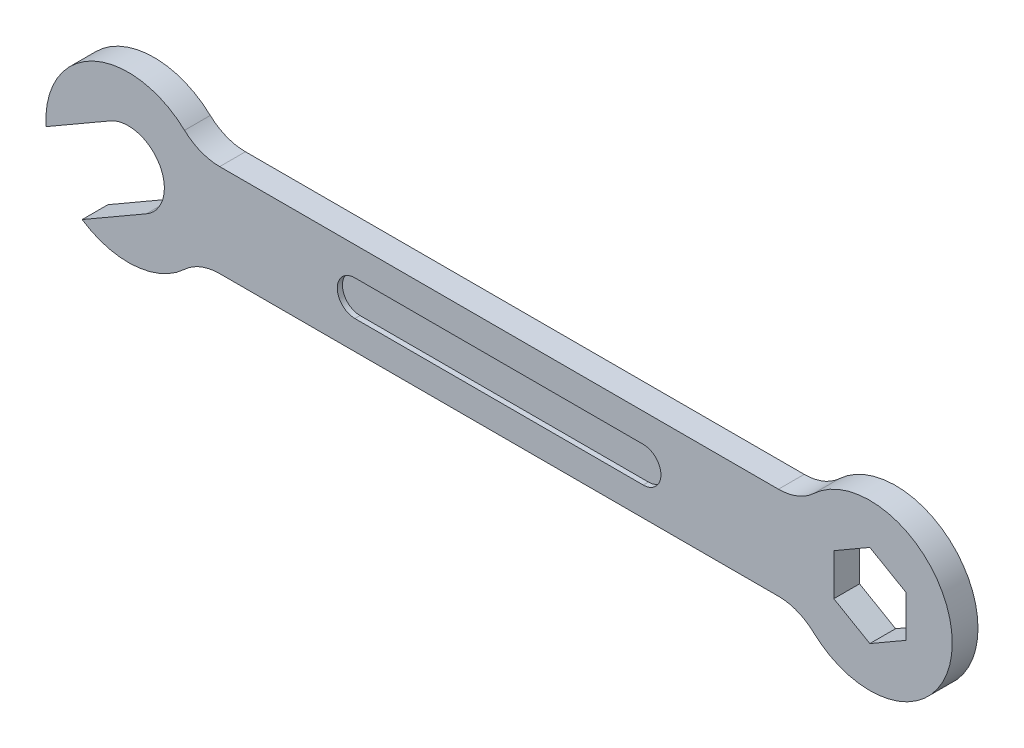
ISO-10303-21;
HEADER;
FILE_DESCRIPTION(('STEP AP214'),'2;1');
FILE_NAME('part.step','',(''),(''),'','','');
FILE_SCHEMA(('AUTOMOTIVE_DESIGN { 1 0 10303 214 1 1 1 1 }'));
ENDSEC;
DATA;
#1=APPLICATION_CONTEXT('core data for automotive mechanical design processes');
#2=APPLICATION_PROTOCOL_DEFINITION('international standard','automotive_design',2000,#1);
#3=PRODUCT_CONTEXT('',#1,'mechanical');
#4=PRODUCT('Part','Part','',(#3));
#5=PRODUCT_RELATED_PRODUCT_CATEGORY('part','',(#4));
#6=PRODUCT_DEFINITION_FORMATION('','',#4);
#7=PRODUCT_DEFINITION_CONTEXT('part definition',#1,'design');
#8=PRODUCT_DEFINITION('design','',#6,#7);
#9=PRODUCT_DEFINITION_SHAPE('','',#8);
#10=(LENGTH_UNIT() NAMED_UNIT(*) SI_UNIT(.MILLI.,.METRE.));
#11=(NAMED_UNIT(*) PLANE_ANGLE_UNIT() SI_UNIT($,.RADIAN.));
#12=(NAMED_UNIT(*) SI_UNIT($,.STERADIAN.) SOLID_ANGLE_UNIT());
#13=UNCERTAINTY_MEASURE_WITH_UNIT(LENGTH_MEASURE(1.E-05),#10,'distance_accuracy_value','');
#14=(GEOMETRIC_REPRESENTATION_CONTEXT(3) GLOBAL_UNCERTAINTY_ASSIGNED_CONTEXT((#13)) GLOBAL_UNIT_ASSIGNED_CONTEXT((#10,
#11,#12)) REPRESENTATION_CONTEXT('',''));
#15=CARTESIAN_POINT('',(0.,0.,0.));
#16=DIRECTION('',(0.,0.,1.));
#17=DIRECTION('',(1.,0.,0.));
#18=AXIS2_PLACEMENT_3D('',#15,#16,#17);
#19=CARTESIAN_POINT('',(0.,0.,2.5));
#20=DIRECTION('',(0.,0.,1.));
#21=DIRECTION('',(1.,0.,0.));
#22=AXIS2_PLACEMENT_3D('',#19,#20,#21);
#23=PLANE('',#22);
#24=CARTESIAN_POINT('',(22.,0.,2.5));
#25=DIRECTION('',(0.,0.,1.));
#26=DIRECTION('',(1.,0.,0.));
#27=AXIS2_PLACEMENT_3D('',#24,#25,#26);
#28=CIRCLE('',#27,1.71110999045574);
#29=CARTESIAN_POINT('',(22.,1.71110999045574,2.5));
#30=VERTEX_POINT('',#29);
#31=CARTESIAN_POINT('',(22.,-1.71110999045574,2.5));
#32=VERTEX_POINT('',#31);
#33=EDGE_CURVE('E53',#30,#32,#28,.T.);
#34=ORIENTED_EDGE('',*,*,#33,.F.);
#35=DIRECTION('',(-1.,0.,0.));
#36=VECTOR('',#35,1.);
#37=CARTESIAN_POINT('',(22.,1.71110999045574,2.5));
#38=LINE('',#37,#36);
#39=CARTESIAN_POINT('',(50.,1.71110999045574,2.5));
#40=VERTEX_POINT('',#39);
#41=EDGE_CURVE('E208',#40,#30,#38,.T.);
#42=ORIENTED_EDGE('',*,*,#41,.F.);
#43=CARTESIAN_POINT('',(50.,0.,2.5));
#44=DIRECTION('',(0.,0.,1.));
#45=DIRECTION('',(1.,0.,0.));
#46=AXIS2_PLACEMENT_3D('',#43,#44,#45);
#47=CIRCLE('',#46,1.71110999045574);
#48=CARTESIAN_POINT('',(50.,-1.71110999045574,2.5));
#49=VERTEX_POINT('',#48);
#50=EDGE_CURVE('E211',#49,#40,#47,.T.);
#51=ORIENTED_EDGE('',*,*,#50,.F.);
#52=DIRECTION('',(1.,0.,0.));
#53=VECTOR('',#52,1.);
#54=CARTESIAN_POINT('',(22.,-1.71110999045574,2.5));
#55=LINE('',#54,#53);
#56=EDGE_CURVE('E220',#32,#49,#55,.T.);
#57=ORIENTED_EDGE('',*,*,#56,.F.);
#58=EDGE_LOOP('',(#34,#42,#51,#57));
#59=FACE_BOUND('',#58,.T.);
#60=CARTESIAN_POINT('',(0.,0.,2.5));
#61=DIRECTION('',(0.,0.,-1.));
#62=DIRECTION('',(1.,0.,0.));
#63=AXIS2_PLACEMENT_3D('',#60,#61,#62);
#64=CIRCLE('',#63,3.5);
#65=CARTESIAN_POINT('',(-1.75,3.03108891324553,2.5));
#66=VERTEX_POINT('',#65);
#67=CARTESIAN_POINT('',(1.75,-3.03108891324553,2.5));
#68=VERTEX_POINT('',#67);
#69=EDGE_CURVE('E269',#66,#68,#64,.T.);
#70=ORIENTED_EDGE('',*,*,#69,.T.);
#71=DIRECTION('',(-0.866025403784438,-0.500000000000001,0.));
#72=VECTOR('',#71,1.);
#73=CARTESIAN_POINT('',(1.75,-3.03108891324553,2.5));
#74=LINE('',#73,#72);
#75=CARTESIAN_POINT('',(-4.47996789718855,-6.62796255573008,2.5));
#76=VERTEX_POINT('',#75);
#77=EDGE_CURVE('E272',#68,#76,#74,.T.);
#78=ORIENTED_EDGE('',*,*,#77,.T.);
#79=CARTESIAN_POINT('',(0.,0.,2.5));
#80=DIRECTION('',(0.,0.,1.));
#81=DIRECTION('',(1.,0.,0.));
#82=AXIS2_PLACEMENT_3D('',#79,#80,#81);
#83=CIRCLE('',#82,8.);
#84=CARTESIAN_POINT('',(5.46099672286118,-5.84615384615385,2.5));
#85=VERTEX_POINT('',#84);
#86=EDGE_CURVE('E277',#76,#85,#83,.T.);
#87=ORIENTED_EDGE('',*,*,#86,.T.);
#88=CARTESIAN_POINT('',(8.87411967464942,-9.5,2.5));
#89=DIRECTION('',(0.,0.,-1.));
#90=DIRECTION('',(1.,0.,0.));
#91=AXIS2_PLACEMENT_3D('',#88,#89,#90);
#92=CIRCLE('',#91,5.);
#93=CARTESIAN_POINT('',(8.87411967464942,-4.5,2.5));
#94=VERTEX_POINT('',#93);
#95=EDGE_CURVE('E279',#85,#94,#92,.T.);
#96=ORIENTED_EDGE('',*,*,#95,.T.);
#97=DIRECTION('',(1.,0.,0.));
#98=VECTOR('',#97,1.);
#99=CARTESIAN_POINT('',(8.87411967464942,-4.5,2.5));
#100=LINE('',#99,#98);
#101=CARTESIAN_POINT('',(63.1258803253506,-4.5,2.5));
#102=VERTEX_POINT('',#101);
#103=EDGE_CURVE('E278',#94,#102,#100,.T.);
#104=ORIENTED_EDGE('',*,*,#103,.T.);
#105=CARTESIAN_POINT('',(63.1258803253506,-9.50000000000001,2.5));
#106=DIRECTION('',(0.,0.,-1.));
#107=DIRECTION('',(1.,0.,0.));
#108=AXIS2_PLACEMENT_3D('',#105,#106,#107);
#109=CIRCLE('',#108,5.00000000000001);
#110=CARTESIAN_POINT('',(66.5390032771388,-5.84615384615384,2.5));
#111=VERTEX_POINT('',#110);
#112=EDGE_CURVE('E281',#102,#111,#109,.T.);
#113=ORIENTED_EDGE('',*,*,#112,.T.);
#114=CARTESIAN_POINT('',(72.,0.,2.5));
#115=DIRECTION('',(0.,0.,1.));
#116=DIRECTION('',(1.,0.,0.));
#117=AXIS2_PLACEMENT_3D('',#114,#115,#116);
#118=CIRCLE('',#117,7.99999999999999);
#119=CARTESIAN_POINT('',(66.5390032771388,5.84615384615385,2.5));
#120=VERTEX_POINT('',#119);
#121=EDGE_CURVE('E283',#111,#120,#118,.T.);
#122=ORIENTED_EDGE('',*,*,#121,.T.);
#123=CARTESIAN_POINT('',(63.1258803253506,9.50000000000001,2.5));
#124=DIRECTION('',(0.,0.,-1.));
#125=DIRECTION('',(1.,0.,0.));
#126=AXIS2_PLACEMENT_3D('',#123,#124,#125);
#127=CIRCLE('',#126,5.00000000000001);
#128=CARTESIAN_POINT('',(63.1258803253506,4.5,2.5));
#129=VERTEX_POINT('',#128);
#130=EDGE_CURVE('E289',#120,#129,#127,.T.);
#131=ORIENTED_EDGE('',*,*,#130,.T.);
#132=DIRECTION('',(-1.,0.,0.));
#133=VECTOR('',#132,1.);
#134=CARTESIAN_POINT('',(8.87411967464942,4.5,2.5));
#135=LINE('',#134,#133);
#136=CARTESIAN_POINT('',(8.87411967464942,4.5,2.5));
#137=VERTEX_POINT('',#136);
#138=EDGE_CURVE('E290',#129,#137,#135,.T.);
#139=ORIENTED_EDGE('',*,*,#138,.T.);
#140=CARTESIAN_POINT('',(8.87411967464942,9.5,2.5));
#141=DIRECTION('',(0.,0.,-1.));
#142=DIRECTION('',(1.,0.,0.));
#143=AXIS2_PLACEMENT_3D('',#140,#141,#142);
#144=CIRCLE('',#143,5.);
#145=CARTESIAN_POINT('',(5.46099672286118,5.84615384615385,2.5));
#146=VERTEX_POINT('',#145);
#147=EDGE_CURVE('E287',#137,#146,#144,.T.);
#148=ORIENTED_EDGE('',*,*,#147,.T.);
#149=CARTESIAN_POINT('',(0.,0.,2.5));
#150=DIRECTION('',(0.,0.,1.));
#151=DIRECTION('',(1.,0.,0.));
#152=AXIS2_PLACEMENT_3D('',#149,#150,#151);
#153=CIRCLE('',#152,8.);
#154=CARTESIAN_POINT('',(-7.97996789718856,-0.565784729239017,2.5));
#155=VERTEX_POINT('',#154);
#156=EDGE_CURVE('E295',#146,#155,#153,.T.);
#157=ORIENTED_EDGE('',*,*,#156,.T.);
#158=DIRECTION('',(0.866025403784438,0.500000000000001,0.));
#159=VECTOR('',#158,1.);
#160=CARTESIAN_POINT('',(-1.75,3.03108891324553,2.5));
#161=LINE('',#160,#159);
#162=EDGE_CURVE('E294',#155,#66,#161,.T.);
#163=ORIENTED_EDGE('',*,*,#162,.T.);
#164=EDGE_LOOP('',(#70,#78,#87,#96,#104,#113,#122,#131,#139,#148,#157,#163));
#165=FACE_BOUND('',#164,.T.);
#166=DIRECTION('',(0.,1.,0.));
#167=VECTOR('',#166,1.);
#168=CARTESIAN_POINT('',(75.5,-2.02072594216369,2.5));
#169=LINE('',#168,#167);
#170=CARTESIAN_POINT('',(75.5,-2.02072594216369,2.5));
#171=VERTEX_POINT('',#170);
#172=CARTESIAN_POINT('',(75.5,2.02072594216369,2.5));
#173=VERTEX_POINT('',#172);
#174=EDGE_CURVE('E228',#171,#173,#169,.T.);
#175=ORIENTED_EDGE('',*,*,#174,.F.);
#176=DIRECTION('',(0.866025403784438,0.5,0.));
#177=VECTOR('',#176,1.);
#178=CARTESIAN_POINT('',(72.,-4.04145188432738,2.5));
#179=LINE('',#178,#177);
#180=CARTESIAN_POINT('',(72.,-4.04145188432738,2.5));
#181=VERTEX_POINT('',#180);
#182=EDGE_CURVE('E226',#181,#171,#179,.T.);
#183=ORIENTED_EDGE('',*,*,#182,.F.);
#184=DIRECTION('',(0.866025403784439,-0.5,0.));
#185=VECTOR('',#184,1.);
#186=CARTESIAN_POINT('',(68.5,-2.02072594216369,2.5));
#187=LINE('',#186,#185);
#188=CARTESIAN_POINT('',(68.5,-2.02072594216369,2.5));
#189=VERTEX_POINT('',#188);
#190=EDGE_CURVE('E236',#189,#181,#187,.T.);
#191=ORIENTED_EDGE('',*,*,#190,.F.);
#192=DIRECTION('',(0.,-1.,0.));
#193=VECTOR('',#192,1.);
#194=CARTESIAN_POINT('',(68.5,2.02072594216368,2.5));
#195=LINE('',#194,#193);
#196=CARTESIAN_POINT('',(68.5,2.02072594216368,2.5));
#197=VERTEX_POINT('',#196);
#198=EDGE_CURVE('E237',#197,#189,#195,.T.);
#199=ORIENTED_EDGE('',*,*,#198,.F.);
#200=DIRECTION('',(-0.866025403784438,-0.5,0.));
#201=VECTOR('',#200,1.);
#202=CARTESIAN_POINT('',(72.,4.04145188432738,2.5));
#203=LINE('',#202,#201);
#204=CARTESIAN_POINT('',(72.,4.04145188432738,2.5));
#205=VERTEX_POINT('',#204);
#206=EDGE_CURVE('E233',#205,#197,#203,.T.);
#207=ORIENTED_EDGE('',*,*,#206,.F.);
#208=DIRECTION('',(-0.866025403784439,0.5,0.));
#209=VECTOR('',#208,1.);
#210=CARTESIAN_POINT('',(75.5,2.02072594216369,2.5));
#211=LINE('',#210,#209);
#212=EDGE_CURVE('E231',#173,#205,#211,.T.);
#213=ORIENTED_EDGE('',*,*,#212,.F.);
#214=EDGE_LOOP('',(#175,#183,#191,#199,#207,#213));
#215=FACE_BOUND('',#214,.T.);
#216=ADVANCED_FACE('F39',(#59,#165,#215),#23,.T.);
#217=CARTESIAN_POINT('',(0.,0.,0.));
#218=DIRECTION('',(0.,0.,1.));
#219=DIRECTION('',(1.,0.,0.));
#220=AXIS2_PLACEMENT_3D('',#217,#218,#219);
#221=PLANE('',#220);
#222=CARTESIAN_POINT('',(0.,0.,0.));
#223=DIRECTION('',(0.,0.,-1.));
#224=DIRECTION('',(1.,0.,0.));
#225=AXIS2_PLACEMENT_3D('',#222,#223,#224);
#226=CIRCLE('',#225,3.5);
#227=CARTESIAN_POINT('',(-1.75,3.03108891324553,0.));
#228=VERTEX_POINT('',#227);
#229=CARTESIAN_POINT('',(1.75,-3.03108891324553,0.));
#230=VERTEX_POINT('',#229);
#231=EDGE_CURVE('E267',#228,#230,#226,.T.);
#232=ORIENTED_EDGE('',*,*,#231,.F.);
#233=DIRECTION('',(0.866025403784438,0.500000000000001,0.));
#234=VECTOR('',#233,1.);
#235=CARTESIAN_POINT('',(-1.75,3.03108891324553,0.));
#236=LINE('',#235,#234);
#237=CARTESIAN_POINT('',(-7.97996789718856,-0.565784729239017,0.));
#238=VERTEX_POINT('',#237);
#239=EDGE_CURVE('E273',#238,#228,#236,.T.);
#240=ORIENTED_EDGE('',*,*,#239,.F.);
#241=CARTESIAN_POINT('',(0.,0.,0.));
#242=DIRECTION('',(0.,0.,1.));
#243=DIRECTION('',(1.,0.,0.));
#244=AXIS2_PLACEMENT_3D('',#241,#242,#243);
#245=CIRCLE('',#244,8.);
#246=CARTESIAN_POINT('',(5.46099672286118,5.84615384615385,0.));
#247=VERTEX_POINT('',#246);
#248=EDGE_CURVE('E320',#247,#238,#245,.T.);
#249=ORIENTED_EDGE('',*,*,#248,.F.);
#250=CARTESIAN_POINT('',(8.87411967464942,9.5,0.));
#251=DIRECTION('',(0.,0.,-1.));
#252=DIRECTION('',(1.,0.,0.));
#253=AXIS2_PLACEMENT_3D('',#250,#251,#252);
#254=CIRCLE('',#253,5.);
#255=CARTESIAN_POINT('',(8.87411967464942,4.5,0.));
#256=VERTEX_POINT('',#255);
#257=EDGE_CURVE('E312',#256,#247,#254,.T.);
#258=ORIENTED_EDGE('',*,*,#257,.F.);
#259=DIRECTION('',(-1.,0.,0.));
#260=VECTOR('',#259,1.);
#261=CARTESIAN_POINT('',(8.87411967464942,4.5,0.));
#262=LINE('',#261,#260);
#263=CARTESIAN_POINT('',(63.1258803253506,4.5,0.));
#264=VERTEX_POINT('',#263);
#265=EDGE_CURVE('E311',#264,#256,#262,.T.);
#266=ORIENTED_EDGE('',*,*,#265,.F.);
#267=CARTESIAN_POINT('',(63.1258803253506,9.50000000000001,0.));
#268=DIRECTION('',(0.,0.,-1.));
#269=DIRECTION('',(1.,0.,0.));
#270=AXIS2_PLACEMENT_3D('',#267,#268,#269);
#271=CIRCLE('',#270,5.00000000000001);
#272=CARTESIAN_POINT('',(66.5390032771388,5.84615384615385,0.));
#273=VERTEX_POINT('',#272);
#274=EDGE_CURVE('E313',#273,#264,#271,.T.);
#275=ORIENTED_EDGE('',*,*,#274,.F.);
#276=CARTESIAN_POINT('',(72.,0.,0.));
#277=DIRECTION('',(0.,0.,1.));
#278=DIRECTION('',(1.,0.,0.));
#279=AXIS2_PLACEMENT_3D('',#276,#277,#278);
#280=CIRCLE('',#279,7.99999999999999);
#281=CARTESIAN_POINT('',(66.5390032771388,-5.84615384615384,0.));
#282=VERTEX_POINT('',#281);
#283=EDGE_CURVE('E310',#282,#273,#280,.T.);
#284=ORIENTED_EDGE('',*,*,#283,.F.);
#285=CARTESIAN_POINT('',(63.1258803253506,-9.50000000000001,0.));
#286=DIRECTION('',(0.,0.,-1.));
#287=DIRECTION('',(1.,0.,0.));
#288=AXIS2_PLACEMENT_3D('',#285,#286,#287);
#289=CIRCLE('',#288,5.00000000000001);
#290=CARTESIAN_POINT('',(63.1258803253506,-4.5,0.));
#291=VERTEX_POINT('',#290);
#292=EDGE_CURVE('E307',#291,#282,#289,.T.);
#293=ORIENTED_EDGE('',*,*,#292,.F.);
#294=DIRECTION('',(1.,0.,0.));
#295=VECTOR('',#294,1.);
#296=CARTESIAN_POINT('',(8.87411967464942,-4.5,0.));
#297=LINE('',#296,#295);
#298=CARTESIAN_POINT('',(8.87411967464942,-4.5,0.));
#299=VERTEX_POINT('',#298);
#300=EDGE_CURVE('E302',#299,#291,#297,.T.);
#301=ORIENTED_EDGE('',*,*,#300,.F.);
#302=CARTESIAN_POINT('',(8.87411967464942,-9.5,0.));
#303=DIRECTION('',(0.,0.,-1.));
#304=DIRECTION('',(1.,0.,0.));
#305=AXIS2_PLACEMENT_3D('',#302,#303,#304);
#306=CIRCLE('',#305,5.);
#307=CARTESIAN_POINT('',(5.46099672286118,-5.84615384615385,0.));
#308=VERTEX_POINT('',#307);
#309=EDGE_CURVE('E305',#308,#299,#306,.T.);
#310=ORIENTED_EDGE('',*,*,#309,.F.);
#311=CARTESIAN_POINT('',(0.,0.,0.));
#312=DIRECTION('',(0.,0.,1.));
#313=DIRECTION('',(1.,0.,0.));
#314=AXIS2_PLACEMENT_3D('',#311,#312,#313);
#315=CIRCLE('',#314,8.);
#316=CARTESIAN_POINT('',(-4.47996789718855,-6.62796255573008,0.));
#317=VERTEX_POINT('',#316);
#318=EDGE_CURVE('E304',#317,#308,#315,.T.);
#319=ORIENTED_EDGE('',*,*,#318,.F.);
#320=DIRECTION('',(-0.866025403784438,-0.500000000000001,0.));
#321=VECTOR('',#320,1.);
#322=CARTESIAN_POINT('',(1.75,-3.03108891324553,0.));
#323=LINE('',#322,#321);
#324=EDGE_CURVE('E298',#230,#317,#323,.T.);
#325=ORIENTED_EDGE('',*,*,#324,.F.);
#326=EDGE_LOOP('',(#232,#240,#249,#258,#266,#275,#284,#293,#301,#310,#319,#325));
#327=FACE_BOUND('',#326,.T.);
#328=DIRECTION('',(0.866025403784438,0.5,0.));
#329=VECTOR('',#328,1.);
#330=CARTESIAN_POINT('',(72.,-4.04145188432738,0.));
#331=LINE('',#330,#329);
#332=CARTESIAN_POINT('',(72.,-4.04145188432738,0.));
#333=VERTEX_POINT('',#332);
#334=CARTESIAN_POINT('',(75.5,-2.02072594216369,0.));
#335=VERTEX_POINT('',#334);
#336=EDGE_CURVE('E224',#333,#335,#331,.T.);
#337=ORIENTED_EDGE('',*,*,#336,.T.);
#338=DIRECTION('',(0.,1.,0.));
#339=VECTOR('',#338,1.);
#340=CARTESIAN_POINT('',(75.5,-2.02072594216369,0.));
#341=LINE('',#340,#339);
#342=CARTESIAN_POINT('',(75.5,2.02072594216369,0.));
#343=VERTEX_POINT('',#342);
#344=EDGE_CURVE('E245',#335,#343,#341,.T.);
#345=ORIENTED_EDGE('',*,*,#344,.T.);
#346=DIRECTION('',(-0.866025403784439,0.5,0.));
#347=VECTOR('',#346,1.);
#348=CARTESIAN_POINT('',(75.5,2.02072594216369,0.));
#349=LINE('',#348,#347);
#350=CARTESIAN_POINT('',(72.,4.04145188432738,0.));
#351=VERTEX_POINT('',#350);
#352=EDGE_CURVE('E249',#343,#351,#349,.T.);
#353=ORIENTED_EDGE('',*,*,#352,.T.);
#354=DIRECTION('',(-0.866025403784438,-0.5,0.));
#355=VECTOR('',#354,1.);
#356=CARTESIAN_POINT('',(72.,4.04145188432738,0.));
#357=LINE('',#356,#355);
#358=CARTESIAN_POINT('',(68.5,2.02072594216368,0.));
#359=VERTEX_POINT('',#358);
#360=EDGE_CURVE('E248',#351,#359,#357,.T.);
#361=ORIENTED_EDGE('',*,*,#360,.T.);
#362=DIRECTION('',(0.,-1.,0.));
#363=VECTOR('',#362,1.);
#364=CARTESIAN_POINT('',(68.5,2.02072594216368,0.));
#365=LINE('',#364,#363);
#366=CARTESIAN_POINT('',(68.5,-2.02072594216369,0.));
#367=VERTEX_POINT('',#366);
#368=EDGE_CURVE('E252',#359,#367,#365,.T.);
#369=ORIENTED_EDGE('',*,*,#368,.T.);
#370=DIRECTION('',(0.866025403784439,-0.5,0.));
#371=VECTOR('',#370,1.);
#372=CARTESIAN_POINT('',(68.5,-2.02072594216369,0.));
#373=LINE('',#372,#371);
#374=EDGE_CURVE('E227',#367,#333,#373,.T.);
#375=ORIENTED_EDGE('',*,*,#374,.T.);
#376=EDGE_LOOP('',(#337,#345,#353,#361,#369,#375));
#377=FACE_BOUND('',#376,.T.);
#378=ADVANCED_FACE('F358',(#327,#377),#221,.F.);
#379=CARTESIAN_POINT('',(0.,0.,2.5));
#380=DIRECTION('',(0.,0.,-1.));
#381=DIRECTION('',(-1.,0.,0.));
#382=AXIS2_PLACEMENT_3D('',#379,#380,#381);
#383=CYLINDRICAL_SURFACE('',#382,3.5);
#384=ORIENTED_EDGE('',*,*,#231,.T.);
#385=DIRECTION('',(0.,0.,-1.));
#386=VECTOR('',#385,1.);
#387=CARTESIAN_POINT('',(1.75,-3.03108891324553,2.5));
#388=LINE('',#387,#386);
#389=EDGE_CURVE('E11',#68,#230,#388,.T.);
#390=ORIENTED_EDGE('',*,*,#389,.F.);
#391=ORIENTED_EDGE('',*,*,#69,.F.);
#392=DIRECTION('',(0.,0.,-1.));
#393=VECTOR('',#392,1.);
#394=CARTESIAN_POINT('',(-1.75,3.03108891324553,2.5));
#395=LINE('',#394,#393);
#396=EDGE_CURVE('E299',#66,#228,#395,.T.);
#397=ORIENTED_EDGE('',*,*,#396,.T.);
#398=EDGE_LOOP('',(#384,#390,#391,#397));
#399=FACE_BOUND('',#398,.T.);
#400=ADVANCED_FACE('F41',(#399),#383,.F.);
#401=CARTESIAN_POINT('',(1.75,-3.03108891324553,2.5));
#402=DIRECTION('',(0.500000000000001,-0.866025403784438,0.));
#403=DIRECTION('',(0.866025403784438,0.500000000000001,0.));
#404=AXIS2_PLACEMENT_3D('',#401,#402,#403);
#405=PLANE('',#404);
#406=ORIENTED_EDGE('',*,*,#324,.T.);
#407=DIRECTION('',(0.,0.,-1.));
#408=VECTOR('',#407,1.);
#409=CARTESIAN_POINT('',(-4.47996789718855,-6.62796255573008,2.5));
#410=LINE('',#409,#408);
#411=EDGE_CURVE('E50',#76,#317,#410,.T.);
#412=ORIENTED_EDGE('',*,*,#411,.F.);
#413=ORIENTED_EDGE('',*,*,#77,.F.);
#414=ORIENTED_EDGE('',*,*,#389,.T.);
#415=EDGE_LOOP('',(#406,#412,#413,#414));
#416=FACE_BOUND('',#415,.T.);
#417=ADVANCED_FACE('F380',(#416),#405,.F.);
#418=CARTESIAN_POINT('',(0.,0.,2.5));
#419=DIRECTION('',(0.,0.,-1.));
#420=DIRECTION('',(-1.,0.,0.));
#421=AXIS2_PLACEMENT_3D('',#418,#419,#420);
#422=CYLINDRICAL_SURFACE('',#421,8.);
#423=ORIENTED_EDGE('',*,*,#318,.T.);
#424=DIRECTION('',(0.,0.,-1.));
#425=VECTOR('',#424,1.);
#426=CARTESIAN_POINT('',(5.46099672286118,-5.84615384615385,2.5));
#427=LINE('',#426,#425);
#428=EDGE_CURVE('E347',#85,#308,#427,.T.);
#429=ORIENTED_EDGE('',*,*,#428,.F.);
#430=ORIENTED_EDGE('',*,*,#86,.F.);
#431=ORIENTED_EDGE('',*,*,#411,.T.);
#432=EDGE_LOOP('',(#423,#429,#430,#431));
#433=FACE_BOUND('',#432,.T.);
#434=ADVANCED_FACE('F355',(#433),#422,.T.);
#435=CARTESIAN_POINT('',(8.87411967464942,-9.5,2.5));
#436=DIRECTION('',(0.,0.,-1.));
#437=DIRECTION('',(-1.,0.,0.));
#438=AXIS2_PLACEMENT_3D('',#435,#436,#437);
#439=CYLINDRICAL_SURFACE('',#438,5.);
#440=ORIENTED_EDGE('',*,*,#309,.T.);
#441=DIRECTION('',(0.,0.,-1.));
#442=VECTOR('',#441,1.);
#443=CARTESIAN_POINT('',(8.87411967464942,-4.5,2.5));
#444=LINE('',#443,#442);
#445=EDGE_CURVE('E345',#94,#299,#444,.T.);
#446=ORIENTED_EDGE('',*,*,#445,.F.);
#447=ORIENTED_EDGE('',*,*,#95,.F.);
#448=ORIENTED_EDGE('',*,*,#428,.T.);
#449=EDGE_LOOP('',(#440,#446,#447,#448));
#450=FACE_BOUND('',#449,.T.);
#451=ADVANCED_FACE('F364',(#450),#439,.F.);
#452=CARTESIAN_POINT('',(8.87411967464942,-4.5,2.5));
#453=DIRECTION('',(0.,1.,0.));
#454=DIRECTION('',(-1.,0.,0.));
#455=AXIS2_PLACEMENT_3D('',#452,#453,#454);
#456=PLANE('',#455);
#457=ORIENTED_EDGE('',*,*,#300,.T.);
#458=DIRECTION('',(0.,0.,-1.));
#459=VECTOR('',#458,1.);
#460=CARTESIAN_POINT('',(63.1258803253506,-4.5,2.5));
#461=LINE('',#460,#459);
#462=EDGE_CURVE('E337',#102,#291,#461,.T.);
#463=ORIENTED_EDGE('',*,*,#462,.F.);
#464=ORIENTED_EDGE('',*,*,#103,.F.);
#465=ORIENTED_EDGE('',*,*,#445,.T.);
#466=EDGE_LOOP('',(#457,#463,#464,#465));
#467=FACE_BOUND('',#466,.T.);
#468=ADVANCED_FACE('F369',(#467),#456,.F.);
#469=CARTESIAN_POINT('',(63.1258803253506,-9.50000000000001,2.5));
#470=DIRECTION('',(0.,0.,-1.));
#471=DIRECTION('',(-1.,0.,0.));
#472=AXIS2_PLACEMENT_3D('',#469,#470,#471);
#473=CYLINDRICAL_SURFACE('',#472,5.00000000000001);
#474=ORIENTED_EDGE('',*,*,#292,.T.);
#475=DIRECTION('',(0.,0.,-1.));
#476=VECTOR('',#475,1.);
#477=CARTESIAN_POINT('',(66.5390032771388,-5.84615384615384,2.5));
#478=LINE('',#477,#476);
#479=EDGE_CURVE('E336',#111,#282,#478,.T.);
#480=ORIENTED_EDGE('',*,*,#479,.F.);
#481=ORIENTED_EDGE('',*,*,#112,.F.);
#482=ORIENTED_EDGE('',*,*,#462,.T.);
#483=EDGE_LOOP('',(#474,#480,#481,#482));
#484=FACE_BOUND('',#483,.T.);
#485=ADVANCED_FACE('F407',(#484),#473,.F.);
#486=CARTESIAN_POINT('',(72.,0.,2.5));
#487=DIRECTION('',(0.,0.,-1.));
#488=DIRECTION('',(-1.,0.,0.));
#489=AXIS2_PLACEMENT_3D('',#486,#487,#488);
#490=CYLINDRICAL_SURFACE('',#489,7.99999999999999);
#491=ORIENTED_EDGE('',*,*,#283,.T.);
#492=DIRECTION('',(0.,0.,-1.));
#493=VECTOR('',#492,1.);
#494=CARTESIAN_POINT('',(66.5390032771388,5.84615384615385,2.5));
#495=LINE('',#494,#493);
#496=EDGE_CURVE('E331',#120,#273,#495,.T.);
#497=ORIENTED_EDGE('',*,*,#496,.F.);
#498=ORIENTED_EDGE('',*,*,#121,.F.);
#499=ORIENTED_EDGE('',*,*,#479,.T.);
#500=EDGE_LOOP('',(#491,#497,#498,#499));
#501=FACE_BOUND('',#500,.T.);
#502=ADVANCED_FACE('F410',(#501),#490,.T.);
#503=CARTESIAN_POINT('',(63.1258803253506,9.50000000000001,2.5));
#504=DIRECTION('',(0.,0.,-1.));
#505=DIRECTION('',(-1.,0.,0.));
#506=AXIS2_PLACEMENT_3D('',#503,#504,#505);
#507=CYLINDRICAL_SURFACE('',#506,5.00000000000001);
#508=ORIENTED_EDGE('',*,*,#274,.T.);
#509=DIRECTION('',(0.,0.,-1.));
#510=VECTOR('',#509,1.);
#511=CARTESIAN_POINT('',(63.1258803253506,4.5,2.5));
#512=LINE('',#511,#510);
#513=EDGE_CURVE('E332',#129,#264,#512,.T.);
#514=ORIENTED_EDGE('',*,*,#513,.F.);
#515=ORIENTED_EDGE('',*,*,#130,.F.);
#516=ORIENTED_EDGE('',*,*,#496,.T.);
#517=EDGE_LOOP('',(#508,#514,#515,#516));
#518=FACE_BOUND('',#517,.T.);
#519=ADVANCED_FACE('F404',(#518),#507,.F.);
#520=CARTESIAN_POINT('',(8.87411967464942,4.5,2.5));
#521=DIRECTION('',(0.,-1.,0.));
#522=DIRECTION('',(1.,0.,0.));
#523=AXIS2_PLACEMENT_3D('',#520,#521,#522);
#524=PLANE('',#523);
#525=ORIENTED_EDGE('',*,*,#265,.T.);
#526=DIRECTION('',(0.,0.,-1.));
#527=VECTOR('',#526,1.);
#528=CARTESIAN_POINT('',(8.87411967464942,4.5,2.5));
#529=LINE('',#528,#527);
#530=EDGE_CURVE('E327',#137,#256,#529,.T.);
#531=ORIENTED_EDGE('',*,*,#530,.F.);
#532=ORIENTED_EDGE('',*,*,#138,.F.);
#533=ORIENTED_EDGE('',*,*,#513,.T.);
#534=EDGE_LOOP('',(#525,#531,#532,#533));
#535=FACE_BOUND('',#534,.T.);
#536=ADVANCED_FACE('F398',(#535),#524,.F.);
#537=CARTESIAN_POINT('',(8.87411967464942,9.5,2.5));
#538=DIRECTION('',(0.,0.,-1.));
#539=DIRECTION('',(-1.,0.,0.));
#540=AXIS2_PLACEMENT_3D('',#537,#538,#539);
#541=CYLINDRICAL_SURFACE('',#540,5.);
#542=ORIENTED_EDGE('',*,*,#257,.T.);
#543=DIRECTION('',(0.,0.,-1.));
#544=VECTOR('',#543,1.);
#545=CARTESIAN_POINT('',(5.46099672286118,5.84615384615385,2.5));
#546=LINE('',#545,#544);
#547=EDGE_CURVE('E324',#146,#247,#546,.T.);
#548=ORIENTED_EDGE('',*,*,#547,.F.);
#549=ORIENTED_EDGE('',*,*,#147,.F.);
#550=ORIENTED_EDGE('',*,*,#530,.T.);
#551=EDGE_LOOP('',(#542,#548,#549,#550));
#552=FACE_BOUND('',#551,.T.);
#553=ADVANCED_FACE('F395',(#552),#541,.F.);
#554=CARTESIAN_POINT('',(0.,0.,2.5));
#555=DIRECTION('',(0.,0.,-1.));
#556=DIRECTION('',(-1.,0.,0.));
#557=AXIS2_PLACEMENT_3D('',#554,#555,#556);
#558=CYLINDRICAL_SURFACE('',#557,8.);
#559=ORIENTED_EDGE('',*,*,#248,.T.);
#560=DIRECTION('',(0.,0.,-1.));
#561=VECTOR('',#560,1.);
#562=CARTESIAN_POINT('',(-7.97996789718856,-0.565784729239017,2.5));
#563=LINE('',#562,#561);
#564=EDGE_CURVE('E325',#155,#238,#563,.T.);
#565=ORIENTED_EDGE('',*,*,#564,.F.);
#566=ORIENTED_EDGE('',*,*,#156,.F.);
#567=ORIENTED_EDGE('',*,*,#547,.T.);
#568=EDGE_LOOP('',(#559,#565,#566,#567));
#569=FACE_BOUND('',#568,.T.);
#570=ADVANCED_FACE('F386',(#569),#558,.T.);
#571=CARTESIAN_POINT('',(-1.75,3.03108891324553,2.5));
#572=DIRECTION('',(-0.500000000000001,0.866025403784438,0.));
#573=DIRECTION('',(-0.866025403784438,-0.500000000000001,0.));
#574=AXIS2_PLACEMENT_3D('',#571,#572,#573);
#575=PLANE('',#574);
#576=ORIENTED_EDGE('',*,*,#239,.T.);
#577=ORIENTED_EDGE('',*,*,#396,.F.);
#578=ORIENTED_EDGE('',*,*,#162,.F.);
#579=ORIENTED_EDGE('',*,*,#564,.T.);
#580=EDGE_LOOP('',(#576,#577,#578,#579));
#581=FACE_BOUND('',#580,.T.);
#582=ADVANCED_FACE('F383',(#581),#575,.F.);
#583=CARTESIAN_POINT('',(72.,-4.04145188432738,2.5));
#584=DIRECTION('',(-0.5,0.866025403784439,0.));
#585=DIRECTION('',(-0.866025403784439,-0.5,0.));
#586=AXIS2_PLACEMENT_3D('',#583,#584,#585);
#587=PLANE('',#586);
#588=ORIENTED_EDGE('',*,*,#336,.F.);
#589=DIRECTION('',(0.,0.,-1.));
#590=VECTOR('',#589,1.);
#591=CARTESIAN_POINT('',(72.,-4.04145188432738,2.5));
#592=LINE('',#591,#590);
#593=EDGE_CURVE('E238',#181,#333,#592,.T.);
#594=ORIENTED_EDGE('',*,*,#593,.F.);
#595=ORIENTED_EDGE('',*,*,#182,.T.);
#596=DIRECTION('',(0.,0.,-1.));
#597=VECTOR('',#596,1.);
#598=CARTESIAN_POINT('',(75.5,-2.02072594216369,2.5));
#599=LINE('',#598,#597);
#600=EDGE_CURVE('E266',#171,#335,#599,.T.);
#601=ORIENTED_EDGE('',*,*,#600,.T.);
#602=EDGE_LOOP('',(#588,#594,#595,#601));
#603=FACE_BOUND('',#602,.T.);
#604=ADVANCED_FACE('F427',(#603),#587,.T.);
#605=CARTESIAN_POINT('',(75.5,-2.02072594216369,2.5));
#606=DIRECTION('',(-1.,0.,0.));
#607=DIRECTION('',(0.,0.,1.));
#608=AXIS2_PLACEMENT_3D('',#605,#606,#607);
#609=PLANE('',#608);
#610=ORIENTED_EDGE('',*,*,#344,.F.);
#611=ORIENTED_EDGE('',*,*,#600,.F.);
#612=ORIENTED_EDGE('',*,*,#174,.T.);
#613=DIRECTION('',(0.,0.,-1.));
#614=VECTOR('',#613,1.);
#615=CARTESIAN_POINT('',(75.5,2.02072594216369,2.5));
#616=LINE('',#615,#614);
#617=EDGE_CURVE('E262',#173,#343,#616,.T.);
#618=ORIENTED_EDGE('',*,*,#617,.T.);
#619=EDGE_LOOP('',(#610,#611,#612,#618));
#620=FACE_BOUND('',#619,.T.);
#621=ADVANCED_FACE('F472',(#620),#609,.T.);
#622=CARTESIAN_POINT('',(75.5,2.02072594216369,2.5));
#623=DIRECTION('',(-0.5,-0.866025403784439,0.));
#624=DIRECTION('',(0.866025403784439,-0.5,0.));
#625=AXIS2_PLACEMENT_3D('',#622,#623,#624);
#626=PLANE('',#625);
#627=ORIENTED_EDGE('',*,*,#352,.F.);
#628=ORIENTED_EDGE('',*,*,#617,.F.);
#629=ORIENTED_EDGE('',*,*,#212,.T.);
#630=DIRECTION('',(0.,0.,-1.));
#631=VECTOR('',#630,1.);
#632=CARTESIAN_POINT('',(72.,4.04145188432738,2.5));
#633=LINE('',#632,#631);
#634=EDGE_CURVE('E265',#205,#351,#633,.T.);
#635=ORIENTED_EDGE('',*,*,#634,.T.);
#636=EDGE_LOOP('',(#627,#628,#629,#635));
#637=FACE_BOUND('',#636,.T.);
#638=ADVANCED_FACE('F477',(#637),#626,.T.);
#639=CARTESIAN_POINT('',(72.,4.04145188432738,2.5));
#640=DIRECTION('',(0.5,-0.866025403784439,0.));
#641=DIRECTION('',(0.866025403784439,0.5,0.));
#642=AXIS2_PLACEMENT_3D('',#639,#640,#641);
#643=PLANE('',#642);
#644=ORIENTED_EDGE('',*,*,#360,.F.);
#645=ORIENTED_EDGE('',*,*,#634,.F.);
#646=ORIENTED_EDGE('',*,*,#206,.T.);
#647=DIRECTION('',(0.,0.,-1.));
#648=VECTOR('',#647,1.);
#649=CARTESIAN_POINT('',(68.5,2.02072594216368,2.5));
#650=LINE('',#649,#648);
#651=EDGE_CURVE('E257',#197,#359,#650,.T.);
#652=ORIENTED_EDGE('',*,*,#651,.T.);
#653=EDGE_LOOP('',(#644,#645,#646,#652));
#654=FACE_BOUND('',#653,.T.);
#655=ADVANCED_FACE('F488',(#654),#643,.T.);
#656=CARTESIAN_POINT('',(68.5,2.02072594216368,2.5));
#657=DIRECTION('',(1.,0.,0.));
#658=DIRECTION('',(0.,0.,-1.));
#659=AXIS2_PLACEMENT_3D('',#656,#657,#658);
#660=PLANE('',#659);
#661=ORIENTED_EDGE('',*,*,#368,.F.);
#662=ORIENTED_EDGE('',*,*,#651,.F.);
#663=ORIENTED_EDGE('',*,*,#198,.T.);
#664=DIRECTION('',(0.,0.,-1.));
#665=VECTOR('',#664,1.);
#666=CARTESIAN_POINT('',(68.5,-2.02072594216369,2.5));
#667=LINE('',#666,#665);
#668=EDGE_CURVE('E61',#189,#367,#667,.T.);
#669=ORIENTED_EDGE('',*,*,#668,.T.);
#670=EDGE_LOOP('',(#661,#662,#663,#669));
#671=FACE_BOUND('',#670,.T.);
#672=ADVANCED_FACE('F500',(#671),#660,.T.);
#673=CARTESIAN_POINT('',(68.5,-2.02072594216369,2.5));
#674=DIRECTION('',(0.5,0.866025403784438,0.));
#675=DIRECTION('',(-0.866025403784439,0.5,0.));
#676=AXIS2_PLACEMENT_3D('',#673,#674,#675);
#677=PLANE('',#676);
#678=ORIENTED_EDGE('',*,*,#374,.F.);
#679=ORIENTED_EDGE('',*,*,#668,.F.);
#680=ORIENTED_EDGE('',*,*,#190,.T.);
#681=ORIENTED_EDGE('',*,*,#593,.T.);
#682=EDGE_LOOP('',(#678,#679,#680,#681));
#683=FACE_BOUND('',#682,.T.);
#684=ADVANCED_FACE('F502',(#683),#677,.T.);
#685=CARTESIAN_POINT('',(22.,0.,2.));
#686=DIRECTION('',(0.,0.,1.));
#687=DIRECTION('',(1.,0.,0.));
#688=AXIS2_PLACEMENT_3D('',#685,#686,#687);
#689=CYLINDRICAL_SURFACE('',#688,1.71110999045574);
#690=ORIENTED_EDGE('',*,*,#33,.T.);
#691=DIRECTION('',(0.,0.,1.));
#692=VECTOR('',#691,1.);
#693=CARTESIAN_POINT('',(22.,-1.71110999045574,2.));
#694=LINE('',#693,#692);
#695=CARTESIAN_POINT('',(22.,-1.71110999045574,2.));
#696=VERTEX_POINT('',#695);
#697=EDGE_CURVE('E189',#696,#32,#694,.T.);
#698=ORIENTED_EDGE('',*,*,#697,.F.);
#699=CARTESIAN_POINT('',(22.,0.,2.));
#700=DIRECTION('',(0.,0.,1.));
#701=DIRECTION('',(1.,0.,0.));
#702=AXIS2_PLACEMENT_3D('',#699,#700,#701);
#703=CIRCLE('',#702,1.71110999045574);
#704=CARTESIAN_POINT('',(22.,1.71110999045574,2.));
#705=VERTEX_POINT('',#704);
#706=EDGE_CURVE('E187',#705,#696,#703,.T.);
#707=ORIENTED_EDGE('',*,*,#706,.F.);
#708=DIRECTION('',(0.,0.,1.));
#709=VECTOR('',#708,1.);
#710=CARTESIAN_POINT('',(22.,1.71110999045574,2.));
#711=LINE('',#710,#709);
#712=EDGE_CURVE('E222',#705,#30,#711,.T.);
#713=ORIENTED_EDGE('',*,*,#712,.T.);
#714=EDGE_LOOP('',(#690,#698,#707,#713));
#715=FACE_BOUND('',#714,.T.);
#716=ADVANCED_FACE('F190',(#715),#689,.F.);
#717=CARTESIAN_POINT('',(22.,1.71110999045574,2.));
#718=DIRECTION('',(0.,1.,0.));
#719=DIRECTION('',(0.,0.,1.));
#720=AXIS2_PLACEMENT_3D('',#717,#718,#719);
#721=PLANE('',#720);
#722=ORIENTED_EDGE('',*,*,#41,.T.);
#723=ORIENTED_EDGE('',*,*,#712,.F.);
#724=DIRECTION('',(-1.,0.,0.));
#725=VECTOR('',#724,1.);
#726=CARTESIAN_POINT('',(22.,1.71110999045574,2.));
#727=LINE('',#726,#725);
#728=CARTESIAN_POINT('',(50.,1.71110999045574,2.));
#729=VERTEX_POINT('',#728);
#730=EDGE_CURVE('E198',#729,#705,#727,.T.);
#731=ORIENTED_EDGE('',*,*,#730,.F.);
#732=DIRECTION('',(0.,0.,1.));
#733=VECTOR('',#732,1.);
#734=CARTESIAN_POINT('',(50.,1.71110999045574,2.));
#735=LINE('',#734,#733);
#736=EDGE_CURVE('E221',#729,#40,#735,.T.);
#737=ORIENTED_EDGE('',*,*,#736,.T.);
#738=EDGE_LOOP('',(#722,#723,#731,#737));
#739=FACE_BOUND('',#738,.T.);
#740=ADVANCED_FACE('F525',(#739),#721,.F.);
#741=CARTESIAN_POINT('',(50.,0.,2.));
#742=DIRECTION('',(0.,0.,1.));
#743=DIRECTION('',(1.,0.,0.));
#744=AXIS2_PLACEMENT_3D('',#741,#742,#743);
#745=CYLINDRICAL_SURFACE('',#744,1.71110999045574);
#746=ORIENTED_EDGE('',*,*,#50,.T.);
#747=ORIENTED_EDGE('',*,*,#736,.F.);
#748=CARTESIAN_POINT('',(50.,0.,2.));
#749=DIRECTION('',(0.,0.,1.));
#750=DIRECTION('',(1.,0.,0.));
#751=AXIS2_PLACEMENT_3D('',#748,#749,#750);
#752=CIRCLE('',#751,1.71110999045574);
#753=CARTESIAN_POINT('',(50.,-1.71110999045574,2.));
#754=VERTEX_POINT('',#753);
#755=EDGE_CURVE('E204',#754,#729,#752,.T.);
#756=ORIENTED_EDGE('',*,*,#755,.F.);
#757=DIRECTION('',(0.,0.,1.));
#758=VECTOR('',#757,1.);
#759=CARTESIAN_POINT('',(50.,-1.71110999045574,2.));
#760=LINE('',#759,#758);
#761=EDGE_CURVE('E192',#754,#49,#760,.T.);
#762=ORIENTED_EDGE('',*,*,#761,.T.);
#763=EDGE_LOOP('',(#746,#747,#756,#762));
#764=FACE_BOUND('',#763,.T.);
#765=ADVANCED_FACE('F535',(#764),#745,.F.);
#766=CARTESIAN_POINT('',(22.,-1.71110999045574,2.));
#767=DIRECTION('',(0.,-1.,0.));
#768=DIRECTION('',(0.,0.,-1.));
#769=AXIS2_PLACEMENT_3D('',#766,#767,#768);
#770=PLANE('',#769);
#771=ORIENTED_EDGE('',*,*,#56,.T.);
#772=ORIENTED_EDGE('',*,*,#761,.F.);
#773=DIRECTION('',(1.,0.,0.));
#774=VECTOR('',#773,1.);
#775=CARTESIAN_POINT('',(22.,-1.71110999045574,2.));
#776=LINE('',#775,#774);
#777=EDGE_CURVE('E200',#696,#754,#776,.T.);
#778=ORIENTED_EDGE('',*,*,#777,.F.);
#779=ORIENTED_EDGE('',*,*,#697,.T.);
#780=EDGE_LOOP('',(#771,#772,#778,#779));
#781=FACE_BOUND('',#780,.T.);
#782=ADVANCED_FACE('F199',(#781),#770,.F.);
#783=CARTESIAN_POINT('',(22.,0.,2.));
#784=DIRECTION('',(0.,0.,1.));
#785=DIRECTION('',(1.,0.,0.));
#786=AXIS2_PLACEMENT_3D('',#783,#784,#785);
#787=PLANE('',#786);
#788=ORIENTED_EDGE('',*,*,#706,.T.);
#789=ORIENTED_EDGE('',*,*,#777,.T.);
#790=ORIENTED_EDGE('',*,*,#755,.T.);
#791=ORIENTED_EDGE('',*,*,#730,.T.);
#792=EDGE_LOOP('',(#788,#789,#790,#791));
#793=FACE_BOUND('',#792,.T.);
#794=ADVANCED_FACE('F206',(#793),#787,.T.);
#795=CLOSED_SHELL('',(#216,#378,#400,#417,#434,#451,#468,#485,#502,#519,#536,#553,#570,#582,
#604,#621,#638,#655,#672,#684,#716,#740,#765,#782,#794));
#796=MANIFOLD_SOLID_BREP('B2',#795);
#797=ADVANCED_BREP_SHAPE_REPRESENTATION('',(#18,#796),#14);
#798=SHAPE_DEFINITION_REPRESENTATION(#9,#797);
ENDSEC;
END-ISO-10303-21;
